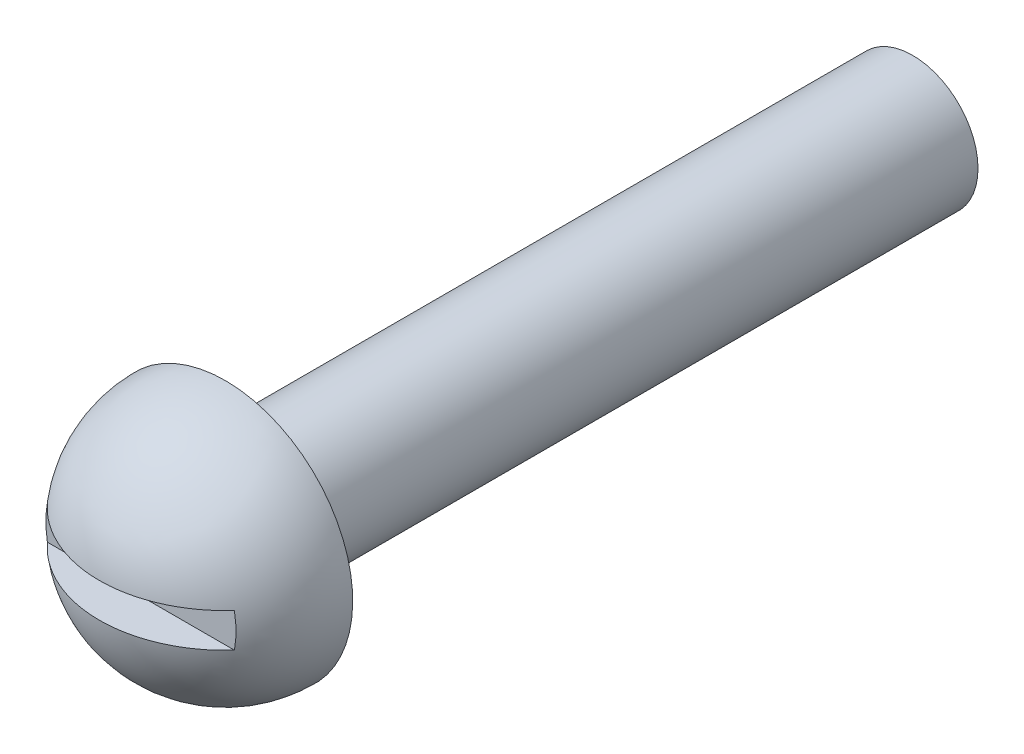
from build123d import *

# Parameters (mm, degrees)
SHANK_PROFILE_0_19_R        = 2.413
SHANK_DEPTH                 = 25.4
SCREWDRIVER_SLOT_DEPTH      = 31.828759505
SCREWDRIVER_SLOT_DEPTH_BACK = 31.828759505
SCREWDRIVER_SLOT_PROFILE_W  = 2.54
SCREWDRIVER_SLOT_PROFILE_H  = 1.27


with BuildPart() as part:
    # Shank Profile Ø0.19 → Shank (new body)
    with BuildSketch(Plane.XY):
        Circle(SHANK_PROFILE_0_19_R)
    extrude(amount=SHANK_DEPTH)

    # Round Head Profile → Round Head (revolve)
    with BuildSketch(Plane(origin=(0, 0, 0), x_dir=(0, 0, -1), z_dir=(1, 0, 0))):
        with BuildLine():
            Line((-25.4, 0), (-25.4, 4.702815049))
            ThreePointArc((-25.4, 4.702815049), (-28.725392412, 3.325392412), (-30.102815049, 0))
            Line((-30.102815049, 0), (-25.4, 0))
        make_face()
    revolve(axis=Axis((0, 0, 25.4), (0, 0, 1)))

    # Screwdriver Slot Profile → Screwdriver Slot (cut, two sides: drawn at the far end of the back side and taken through both)
    with BuildSketch(Plane(origin=(0, 0, 0), x_dir=(0, 0, -1), z_dir=(1, 0, 0)).offset(-SCREWDRIVER_SLOT_DEPTH_BACK)):
        with Locations((-29.795276549, 0)):
            Rectangle(SCREWDRIVER_SLOT_PROFILE_W, SCREWDRIVER_SLOT_PROFILE_H)
    extrude(amount=SCREWDRIVER_SLOT_DEPTH + SCREWDRIVER_SLOT_DEPTH_BACK, mode=Mode.SUBTRACT)


solid = part.part
